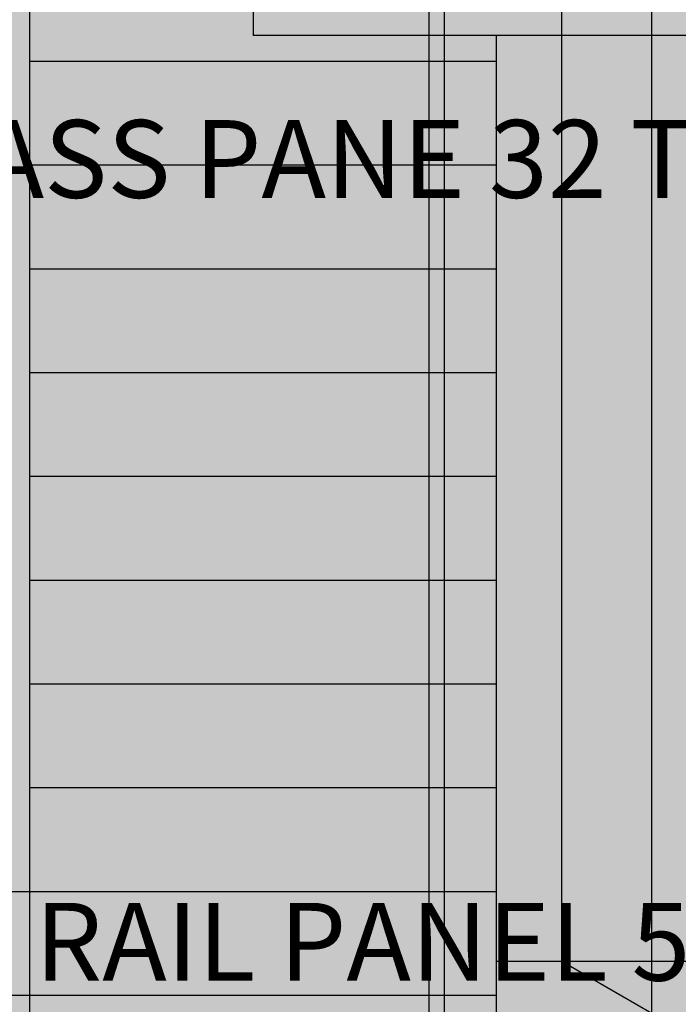
# Model space of a CAD drawing. Units: millimetres. Extents: x 131 to 845, y -20 to 1043.
# Tile 6 of 11: x 368 to 495, y 302 to 492. Entities that reach past the tile are written whole.
import ezdxf

# ---------------------------------------------------------------- set-up
doc = ezdxf.new("R2010")
doc.units = ezdxf.units.MM
doc.header["$MEASUREMENT"] = 0
for name, color, linetype, lineweight in [('A-ANNO-DIMS', 2, 'Continuous', 18), ('A-ELEV', 7, 'Continuous', 25), ('A-ELEV-PATT', 7, 'Continuous', 13), ('A-WALL-PATT', 131, 'Continuous', 13)]:
    doc.layers.add(name, color=color, linetype=linetype, lineweight=lineweight)
doc.styles.get("Standard").update_dxf_attribs({"font": 'arial.ttf'})
doc.dimstyles.get("Standard").update_dxf_attribs({"dimtxt": 15, "dimasz": 10, "dimexe": 0.18, "dimexo": 0.0625, "dimgap": 5, "dimtad": 0, "dimtih": 1, "dimtoh": 1, "dimdec": 0, "dimzin": 0, "dimdsep": 46, "dimtxsty": 'Standard', "dimcen": 5, "dimadec": 0, "dimazin": 0, "dimtfac": 1, "dimtdec": 0, "dimtofl": 0, "dimtmove": 0, "dimatfit": 3, "dimfxl": 1, "dimtolj": 1, "dimtzin": 0, "dimarcsym": 0})

# ---------------------------------------------------------------- blocks, each defined once
blk = doc.blocks.new('*U5')
blk.add_line((0, 90), (0, 0))
blk = doc.blocks.new('*U6')
at = {"layer": 'A-ELEV', "color": 0, "linetype": 'ByBlock', "lineweight": -2, "transparency": 16777216, "rotation": 270}
for p in [(369.56, 483.56), (369.56, 463.56), (369.56, 443.56), (369.56, 423.56), (369.56, 403.56), (369.56, 383.56), (369.56, 363.56), (369.56, 343.56), (369.56, 323.56), (369.56, 303.56)]:
    blk.add_blockref('*U5', p, dxfattribs=at)
blk = doc.blocks.new('*D9')
at = {"layer": 'A-ANNO-DIMS', "color": 0, "lineweight": -2, "transparency": 16777216}
for p, q in [((571.05, 313.91), (561.05, 313.91)), ((581.05, 313.22), (581.05, 314.09)), ((586.05, 313.22), (586.05, 314.09)), ((596.05, 313.91), (606.05, 313.91))]:
    blk.add_line(p, q, dxfattribs=at)
at = {"layer": 'A-ANNO-DIMS', "color": 0, "transparency": 16777216}
for points in [[(571.05, 315.58), (571.05, 312.24), (581.05, 313.91)], [(596.05, 315.58), (596.05, 312.24), (586.05, 313.91)]]:
    blk.add_solid(points, dxfattribs=at)
at = {"layer": 'Defpoints', "color": 0, "transparency": 16777216}
for p in [(581.05, 313.91), (581.05, 313.16), (586.05, 313.16)]:
    blk.add_point(p, dxfattribs=at)
at = {"layer": 'A-ANNO-DIMS', "color": 0, "transparency": 16777216, "insert": (409.24, 313.91), "char_height": 15, "attachment_point": 5}
blk.add_mtext('\\A1;BALCONY RAIL PANEL 5 TYP.', dxfattribs=at)
blk = doc.blocks.new('*D11')
at = {"layer": 'A-ANNO-DIMS', "color": 0, "lineweight": -2, "transparency": 16777216}
for p, q in [((554.73, 464.78), (544.73, 464.78)), ((554.75, 454.78), (554.73, 464.78)), ((550.09, 454.77), (554.93, 454.78)), ((554.78, 433.28), (554.76, 444.78)), ((550.13, 423.27), (554.97, 423.28))]:
    blk.add_line(p, q, dxfattribs=at)
at = {"layer": 'A-ANNO-DIMS', "color": 0, "transparency": 16777216}
for points in [[(556.43, 444.78), (553.1, 444.77), (554.75, 454.78)], [(556.45, 433.28), (553.11, 433.27), (554.79, 423.28)]]:
    blk.add_solid(points, dxfattribs=at)
at = {"layer": 'Defpoints', "color": 0, "transparency": 16777216}
for p in [(550.02, 454.77), (554.75, 454.78), (550.07, 423.27)]:
    blk.add_point(p, dxfattribs=at)
at = {"layer": 'A-ANNO-DIMS', "color": 0, "transparency": 16777216, "insert": (399.96, 464.78), "char_height": 15, "attachment_point": 5}
blk.add_mtext('\\A1;DOOR GLASS PANE 32 TYP.', dxfattribs=at)
blk = doc.blocks.new('*D14')
at = {"layer": 'A-ANNO-DIMS', "color": 0, "lineweight": -2, "transparency": 16777216}
for p, q in [((210.52, 985.67), (162.55, 985.67)), ((162.73, 975.67), (162.73, 524.4)), ((162.73, 47.81), (162.73, 499.08)), ((459.5, 37.81), (162.55, 37.81))]:
    blk.add_line(p, q, dxfattribs=at)
at = {"layer": 'A-ANNO-DIMS', "color": 0, "transparency": 16777216}
for points in [[(161.06, 975.67), (164.4, 975.67), (162.73, 985.67)], [(161.06, 47.81), (164.4, 47.81), (162.73, 37.81)]]:
    blk.add_solid(points, dxfattribs=at)
at = {"layer": 'Defpoints', "color": 0, "transparency": 16777216}
for p in [(162.73, 985.67), (210.58, 985.67), (459.56, 37.81)]:
    blk.add_point(p, dxfattribs=at)
at = {"layer": 'A-ANNO-DIMS', "color": 0, "transparency": 16777216, "insert": (162.73, 511.74), "char_height": 15, "attachment_point": 5}
blk.add_mtext('\\A1;947.9', dxfattribs=at)
blk = doc.blocks.new('*D35')
at = {"layer": 'A-ANNO-DIMS', "color": 0, "lineweight": -2, "transparency": 16777216}
for p, q in [((369.5, 763.56), (162.55, 763.56)), ((162.73, 753.56), (162.73, 536.21)), ((162.73, 293.56), (162.73, 510.9)), ((369.5, 283.56), (162.55, 283.56))]:
    blk.add_line(p, q, dxfattribs=at)
at = {"layer": 'A-ANNO-DIMS', "color": 0, "transparency": 16777216}
for points in [[(161.06, 753.56), (164.4, 753.56), (162.73, 763.56)], [(161.06, 293.56), (164.4, 293.56), (162.73, 283.56)]]:
    blk.add_solid(points, dxfattribs=at)
at = {"layer": 'Defpoints', "color": 0, "transparency": 16777216}
for p in [(162.73, 763.56), (369.56, 763.56), (369.56, 283.56)]:
    blk.add_point(p, dxfattribs=at)
at = {"layer": 'A-ANNO-DIMS', "color": 0, "transparency": 16777216, "insert": (162.73, 523.56), "char_height": 15, "attachment_point": 5}
blk.add_mtext('\\A1;480', dxfattribs=at)
blk = doc.blocks.new('*D36')
at = {"layer": 'A-ANNO-DIMS', "color": 0, "lineweight": -2, "transparency": 16777216}
for p, q in [((162.73, 333.56), (162.73, 343.56)), ((162.73, 343.56), (172.73, 343.56)), ((369.5, 323.56), (162.55, 323.56)), ((369.5, 303.56), (162.55, 303.56)), ((162.73, 293.56), (162.73, 283.56))]:
    blk.add_line(p, q, dxfattribs=at)
at = {"layer": 'A-ANNO-DIMS', "color": 0, "transparency": 16777216}
for points in [[(161.06, 333.56), (164.4, 333.56), (162.73, 323.56)], [(161.06, 293.56), (164.4, 293.56), (162.73, 303.56)]]:
    blk.add_solid(points, dxfattribs=at)
at = {"layer": 'Defpoints', "color": 0, "transparency": 16777216}
for p in [(162.73, 323.56), (369.56, 323.56), (369.56, 303.56)]:
    blk.add_point(p, dxfattribs=at)
at = {"layer": 'A-ANNO-DIMS', "color": 0, "transparency": 16777216, "insert": (188.58, 343.56), "char_height": 15, "attachment_point": 5}
blk.add_mtext('\\A1;20', dxfattribs=at)
blk = doc.blocks.new('*D50')
at = {"layer": 'A-ANNO-DIMS', "color": 0, "lineweight": -2, "transparency": 16777216}
for p, q in [((720.6, 488.6), (768.56, 488.6)), ((768.38, 478.6), (768.38, 287.12)), ((768.38, 70.31), (768.38, 261.79)), ((216.3, 60.31), (768.56, 60.31))]:
    blk.add_line(p, q, dxfattribs=at)
at = {"layer": 'A-ANNO-DIMS', "color": 0, "transparency": 16777216}
for points in [[(766.72, 478.6), (770.05, 478.6), (768.38, 488.6)], [(766.72, 70.31), (770.05, 70.31), (768.38, 60.31)]]:
    blk.add_solid(points, dxfattribs=at)
at = {"layer": 'Defpoints', "color": 0, "transparency": 16777216}
for p in [(720.53, 488.6), (768.38, 488.6), (216.23, 60.31)]:
    blk.add_point(p, dxfattribs=at)
at = {"layer": 'A-ANNO-DIMS', "color": 0, "transparency": 16777216, "insert": (768.38, 274.45), "char_height": 15, "attachment_point": 5}
blk.add_mtext('\\A1;428.3', dxfattribs=at)
blk = doc.blocks.new('*D75')
at = {"layer": 'A-ANNO-DIMS', "color": 0, "lineweight": -2, "transparency": 16777216}
for p, q in [((462.24, 1033.52), (452.24, 1033.52)), ((472.24, 310.22), (472.24, 1033.7)), ((489.56, 300.22), (489.56, 1033.7)), ((499.56, 1033.52), (509.56, 1033.52))]:
    blk.add_line(p, q, dxfattribs=at)
at = {"layer": 'A-ANNO-DIMS', "color": 0, "transparency": 16777216}
for points in [[(462.24, 1035.18), (462.24, 1031.85), (472.24, 1033.52)], [(499.56, 1035.18), (499.56, 1031.85), (489.56, 1033.52)]]:
    blk.add_solid(points, dxfattribs=at)
at = {"layer": 'Defpoints', "color": 0, "transparency": 16777216}
for p in [(489.56, 1033.52), (472.24, 310.16), (489.56, 300.16)]:
    blk.add_point(p, dxfattribs=at)
at = {"layer": 'A-ANNO-DIMS', "color": 0, "transparency": 16777216, "insert": (539.08, 1033.52), "char_height": 15, "attachment_point": 5}
blk.add_mtext('\\A1;17.32', dxfattribs=at)
blk = doc.blocks.new('*D76')
at = {"layer": 'A-ANNO-DIMS', "color": 0, "lineweight": -2, "transparency": 16777216}
for p, q in [((768.38, 320.16), (768.38, 330.16)), ((472.3, 310.16), (768.56, 310.16)), ((489.62, 300.16), (768.56, 300.16)), ((768.38, 290.16), (768.38, 280.16)), ((768.38, 280.16), (758.38, 280.16))]:
    blk.add_line(p, q, dxfattribs=at)
at = {"layer": 'A-ANNO-DIMS', "color": 0, "transparency": 16777216}
for points in [[(766.72, 320.16), (770.05, 320.16), (768.38, 310.16)], [(766.72, 290.16), (770.05, 290.16), (768.38, 300.16)]]:
    blk.add_solid(points, dxfattribs=at)
at = {"layer": 'Defpoints', "color": 0, "transparency": 16777216}
for p in [(472.24, 310.16), (489.56, 300.16), (768.38, 300.16)]:
    blk.add_point(p, dxfattribs=at)
at = {"layer": 'A-ANNO-DIMS', "color": 0, "transparency": 16777216, "insert": (743.37, 280.16), "char_height": 15, "attachment_point": 5}
blk.add_mtext('\\A1;10', dxfattribs=at)
blk = doc.blocks.new('*D99')
at = {"layer": 'A-ANNO-DIMS', "color": 0, "lineweight": -2, "transparency": 16777216}
for p, q in [((449.56, 833.53), (449.56, -10.22)), ((446.56, 818.53), (446.56, -10.22)), ((436.56, -10.04), (426.56, -10.04)), ((459.56, -10.04), (469.56, -10.04))]:
    blk.add_line(p, q, dxfattribs=at)
at = {"layer": 'A-ANNO-DIMS', "color": 0, "transparency": 16777216}
for points in [[(436.56, -8.37), (436.56, -11.7), (446.56, -10.04)], [(459.56, -8.37), (459.56, -11.7), (449.56, -10.04)]]:
    blk.add_solid(points, dxfattribs=at)
at = {"layer": 'Defpoints', "color": 0, "transparency": 16777216}
for p in [(449.56, 833.6), (446.56, 818.6), (449.56, -10.04)]:
    blk.add_point(p, dxfattribs=at)
at = {"layer": 'A-ANNO-DIMS', "color": 0, "transparency": 16777216, "insert": (479.47, -10.04), "char_height": 15, "attachment_point": 5}
blk.add_mtext('\\A1;3', dxfattribs=at)

msp = doc.modelspace()

# ---------------------------------------------------------------- hatches: boundary and pattern name
at = {"layer": 'A-ELEV-PATT', "transparency": 33554681}
h = msp.add_hatch(color=256, dxfattribs=at)
h.set_gradient(color1=(147, 149, 152), color2=(192, 192, 192), name='CYLINDER')
h.paths.add_polyline_path([(369.5586, 763.5561), (369.5586, 743.5561), (459.5586, 743.5561), (459.5586, 763.5561)])
h.paths.add_polyline_path([(459.5586, 703.5561), (459.5586, 723.5561), (369.5586, 723.5561), (369.5586, 703.5561)])
h.paths.add_polyline_path([(459.5586, 663.5561), (459.5586, 683.5561), (369.5586, 683.5561), (369.5586, 663.5561)])
h.paths.add_polyline_path([(459.5586, 623.5561), (459.5586, 643.5561), (369.5586, 643.5561), (369.5586, 623.5561)])
h.paths.add_polyline_path([(459.5586, 583.5561), (459.5586, 603.5561), (369.5586, 603.5561), (369.5586, 583.5561)])
h.paths.add_polyline_path([(459.5586, 543.5561), (459.5586, 563.5561), (369.5586, 563.5561), (369.5586, 543.5561)])
h.paths.add_polyline_path([(369.5586, 523.5561), (369.5586, 503.5561), (409.6606, 503.5561), (409.6606, 503.5953), (412.6606, 503.5953), (412.6606, 513.5953), (414.417, 523.5561)])
h.paths.add_polyline_path([(369.5586, 483.5561), (369.5586, 463.5561), (459.5586, 463.5561), (459.5586, 483.5561)])
h.paths.add_polyline_path([(459.5586, 423.5561), (459.5586, 443.5561), (369.5586, 443.5561), (369.5586, 423.5561)])
h.paths.add_polyline_path([(369.5586, 403.5561), (369.5586, 383.5561), (459.5586, 383.5561), (459.5586, 403.5561)])
h.paths.add_polyline_path([(459.5586, 343.5561), (459.5586, 363.5561), (369.5586, 363.5561), (369.5586, 343.5561)])
h.paths.add_polyline_path([(369.5586, 323.5561), (369.5586, 303.5561), (459.5586, 303.5561), (459.5586, 323.5561)])
h = msp.add_hatch(color=256, dxfattribs=at)
h.set_gradient(color1=(147, 149, 152), color2=(192, 192, 192), name='CURVED')
h.paths.add_polyline_path([(369.5586, 743.5561), (369.5586, 723.5561), (459.5586, 723.5561), (459.5586, 743.5561)])
h.paths.add_polyline_path([(369.5586, 703.5561), (369.5586, 683.5561), (459.5586, 683.5561), (459.5586, 703.5561)])
h.paths.add_polyline_path([(459.5586, 643.5561), (459.5586, 663.5561), (369.5586, 663.5561), (369.5586, 643.5561)])
h.paths.add_polyline_path([(459.5586, 603.5561), (459.5586, 623.5561), (369.5586, 623.5561), (369.5586, 603.5561)])
h.paths.add_polyline_path([(369.5586, 583.5561), (369.5586, 563.5561), (459.5586, 563.5561), (459.5586, 583.5561)])
h.paths.add_polyline_path([(369.5586, 543.5561), (369.5586, 523.5561), (459.5586, 523.5561), (459.5586, 543.5561)])
h.paths.add_polyline_path([(459.5586, 483.5561), (459.5586, 488.5953), (412.6606, 488.5953), (412.6606, 498.5953), (409.6606, 498.5953), (409.6606, 503.5561), (369.5586, 503.5561), (369.5586, 483.5561)])
h.paths.add_polyline_path([(369.5586, 463.5561), (369.5586, 443.5561), (459.5586, 443.5561), (459.5586, 463.5561)])
h.paths.add_polyline_path([(369.5586, 423.5561), (369.5586, 403.5561), (459.5586, 403.5561), (459.5586, 423.5561)])
h.paths.add_polyline_path([(369.5586, 383.5561), (369.5586, 363.5561), (459.5586, 363.5561), (459.5586, 383.5561)])
h.paths.add_polyline_path([(369.5586, 343.5561), (369.5586, 323.5561), (459.5586, 323.5561), (459.5586, 343.5561)])
h.paths.add_polyline_path([(369.5586, 303.5561), (369.5586, 283.5561), (459.5586, 283.5561), (459.5586, 303.5561)])
h = msp.add_hatch(color=256, dxfattribs=at)
h.set_gradient(color1=(255, 255, 255), color2=(199, 200, 202), name='INVSPHERICAL')
h.paths.add_polyline_path([(459.5586, 310.1596), (472.2381, 310.1596), (489.5586, 300.1596), (650.5349, 300.1596), (628.8842, 312.6596), (628.8842, 488.5953), (459.5586, 488.5953)])
h.paths.add_polyline_path([(525.0467, 459.8046), (615.0467, 459.8046), (615.0467, 323.1596), (617.0467, 323.1596), (617.0467, 319.1596), (615.0467, 319.1596), (615.0467, 309.1596), (617.0467, 309.1596), (617.0467, 305.1596), (572.0467, 305.1596), (572.0453, 303.6234), (570.0467, 303.6234), (570.0467, 305.1596), (525.0467, 305.1596), (523.0467, 305.1596), (523.0467, 309.1596), (525.0467, 309.1596), (525.0467, 319.1596), (523.0467, 319.1596), (523.0467, 323.1596), (525.0467, 323.1596)], flags=16)
h.paths.add_polyline_path([(530.0467, 454.8046), (550.0467, 454.8046), (550.0467, 423.2044), (530.0467, 423.2044)], flags=0)
h.paths.add_polyline_path([(530.0467, 418.2044), (550.0467, 418.2044), (550.0467, 386.7044), (530.0467, 386.7044)], flags=0)
h.paths.add_polyline_path([(560.0467, 439.8046), (563.0467, 439.8046), (563.0467, 328.8046), (560.0467, 328.8046)], flags=0)
h.paths.add_polyline_path([(530.0467, 381.7044), (550.0467, 381.7044), (550.0467, 350.2044), (530.0467, 350.2044)], flags=0)
h.paths.add_polyline_path([(554.0467, 319.1596), (554.0467, 315.1596), (540.0467, 315.1596), (540.0467, 313.7044), (530.0467, 313.7044), (530.0467, 319.1596)], flags=0)
h.paths.add_polyline_path([(556.0467, 319.1596), (561.0467, 319.1596), (561.0467, 315.1596), (556.0467, 315.1596)], flags=0)
h.paths.add_polyline_path([(563.0467, 319.1596), (568.0467, 319.1596), (568.0467, 315.1596), (563.0467, 315.1596)], flags=0)
h.paths.add_polyline_path([(556.0467, 313.1596), (561.0467, 313.1596), (561.0467, 309.1596), (556.0467, 309.1596)], flags=0)
h.paths.add_polyline_path([(563.0467, 313.1596), (568.0467, 313.1596), (568.0467, 309.1596), (563.0467, 309.1596)], flags=0)
h.paths.add_polyline_path([(574.0467, 319.1596), (579.0467, 319.1596), (579.0467, 315.1596), (574.1854, 315.1596), (574.1854, 313.1596), (579.0467, 313.1596), (579.0467, 309.1596), (574.0467, 309.1596), (574.0467, 313.1596), (574.1854, 315.1596), (574.0467, 315.1596)], flags=0)
h.paths.add_polyline_path([(581.0467, 319.1596), (586.0467, 319.1596), (586.0467, 315.1596), (581.0467, 315.1596)], flags=0)
h.paths.add_polyline_path([(581.0467, 313.1596), (586.0467, 313.1596), (586.0467, 309.1596), (581.0467, 309.1596)], flags=0)
h = msp.add_hatch(color=256, dxfattribs=at)
h.set_gradient(color1=(79, 2, 22), color2=(153, 133, 76), name='SPHERICAL')
h.paths.add_polyline_path([(459.5586, 310.1596), (459.5586, 300.1596), (489.5586, 300.1596), (472.2381, 310.1596)])
h.paths.add_polyline_path([(658.8842, 312.6596), (628.8842, 312.6596), (650.5349, 300.1596), (680.5349, 300.1596)])
at = {"layer": 'A-WALL-PATT'}
h = msp.add_hatch(color=256, dxfattribs=at)
h.dxf.hatch_style = 1
h.paths.add_polyline_path([(449.5586, 833.5953), (451.6297, 835.6663), (451.6297, 885.6663), (466.6297, 885.6663), (466.6297, 891.3345), (330.6595, 891.3345), (330.6595, 856.8345), (292.1595, 856.8345), (292.1595, 798.4332), (336.1595, 798.4332), (336.1595, 178.4332), (246.1595, 178.4332), (246.1595, 798.4332), (290.1595, 798.4332), (290.1595, 856.8345), (259.6595, 856.8345), (255.6595, 860.8345), (255.6595, 927.8345), (290.1595, 927.8345), (290.1595, 960.6663), (216.2327, 960.6663), (216.2327, 60.3131), (459.5586, 60.3131), (459.5586, 97.8131), (459.5586, 252.07), (459.5586, 283.5561), (369.5586, 283.5561), (369.5586, 763.5561), (439.5586, 763.5561), (439.5586, 778.6714), (439.5586, 793.5953), (439.5586, 796.5953), (441.5586, 798.5953), (444.5586, 798.5953), (444.5586, 813.5953), (444.5586, 816.5953), (446.5586, 818.5953), (449.5586, 818.5953)])
h.paths.add_polyline_path([(466.6297, 960.6663), (292.1595, 960.6663), (292.1595, 927.8345), (326.6595, 927.8345), (330.6595, 923.8345), (330.6595, 893.3345), (466.6297, 893.3345)], flags=17)
h.paths.add_polyline_path([(720.5349, 813.5953), (720.5349, 818.5953), (710.5349, 818.5953), (449.5586, 818.5953), (446.5586, 818.5953), (444.5586, 816.5953), (444.5586, 813.5953), (444.5586, 798.5953), (705.5349, 798.5953), (705.5349, 513.5953), (705.5349, 498.5953), (680.5349, 498.5953), (680.5349, 488.5953), (705.5349, 488.5953), (720.5349, 488.5953), (720.5349, 513.5953)])
h.paths.add_polyline_path([(680.5349, 498.5953), (412.6606, 498.5953), (412.6606, 488.5953), (680.5349, 488.5953)])

# ---------------------------------------------------------------- linework, layer by layer
at = {"layer": 'A-ELEV'}
for p, q in [((369.5586, 763.5561), (369.5586, 283.5561)), ((412.6606, 498.5953), (412.6606, 488.5953)), ((705.5349, 488.5953), (412.6606, 488.5953)), ((459.5586, 488.5953), (459.5586, 252.07)), ((459.5586, 310.1596), (472.2381, 310.1596)), ((472.2381, 310.1596), (489.5586, 300.1596))]:
    msp.add_line(p, q, dxfattribs=at)

# ---------------------------------------------------------------- block references
msp.add_blockref('*U6', (0, 0), dxfattribs=at)

# ---------------------------------------------------------------- dimensions: what is measured, and where the dimension line sits
at = {"layer": 'A-ANNO-DIMS'}
for base, p1, p2, override, picture, middle in [((489.5586, 1033.5163), (472.2381, 310.1596), (489.5586, 300.1596), {"dimdec": 2, "dimlfac": 1, "dimrnd": 0, "dimzin": 0, "dimdsep": 46, "dimlunit": 2}, '*D75', (539.0845, 1033.5163)), ((449.5586, -10.0369), (446.5586, 818.5953), (449.5586, 833.5953), {"dimdec": 0, "dimlfac": 1, "dimrnd": 0, "dimzin": 0, "dimdsep": 46, "dimlunit": 2}, '*D99', (479.4699, -10.0369))]:
    dim = msp.add_linear_dim(base=base, p1=p1, p2=p2, dimstyle='Standard', override=override, dxfattribs=at)
    dim.commit()
    dim.dimension.update_dxf_attribs({"geometry": picture, "text_midpoint": middle})
for base, p1, p2, override, picture, middle in [((162.7317, 985.6663), (459.5586, 37.8131), (210.5817, 985.6663), {"dimdec": 1, "dimlfac": 1, "dimrnd": 0, "dimzin": 0, "dimdsep": 46, "dimlunit": 2}, '*D14', (162.7317, 511.7397)), ((162.7317, 763.5561), (369.5586, 283.5561), (369.5586, 763.5561), {"dimdec": 0, "dimlfac": 1, "dimrnd": 0, "dimzin": 0, "dimdsep": 46, "dimlunit": 2}, '*D35', (162.7317, 523.5561)), ((768.3849, 488.5953), (216.2327, 60.3131), (720.5349, 488.5953), {"dimdec": 1, "dimlfac": 1, "dimrnd": 0, "dimzin": 0, "dimdsep": 46, "dimlunit": 2}, '*D50', (768.3849, 274.4542)), ((162.7317, 323.5561), (369.5586, 303.5561), (369.5586, 323.5561), {"dimdec": 0, "dimlfac": 1, "dimrnd": 0, "dimzin": 0, "dimdsep": 46, "dimlunit": 2}, '*D36', (188.5775, 343.5561)), ((768.3849, 300.1596), (472.2381, 310.1596), (489.5586, 300.1596), {"dimdec": 0, "dimlfac": 1, "dimrnd": 0, "dimzin": 0, "dimdsep": 46, "dimlunit": 2}, '*D76', (743.3729, 280.1596))]:
    dim = msp.add_linear_dim(base=base, p1=p1, p2=p2, angle=90, dimstyle='Standard', override=override, dxfattribs=at)
    dim.commit()
    dim.dimension.update_dxf_attribs({"geometry": picture, "text_midpoint": middle})
for base, p1, p2, angle, text, picture, middle in [((554.7491, 454.7757), (550.0694, 423.2689), (550.0241, 454.7689), 90.082356, 'DOOR GLASS PANE <> TYP.', '*D11', (399.9615, 464.7756)), ((581.0467, 313.9096), (586.0467, 313.1596), (581.0467, 313.1596), 180, 'BALCONY RAIL PANEL <> TYP.', '*D9', (409.2391, 313.9096))]:
    dim = msp.add_linear_dim(base=base, p1=p1, p2=p2, angle=angle, text=text, dimstyle='Standard', override={"dimdec": 0, "dimrnd": 0, "dimzin": 0, "dimlunit": 2}, dxfattribs=at)
    dim.commit()
    dim.dimension.update_dxf_attribs({"geometry": picture, "text_midpoint": middle})

doc.saveas('drawing.dxf')
